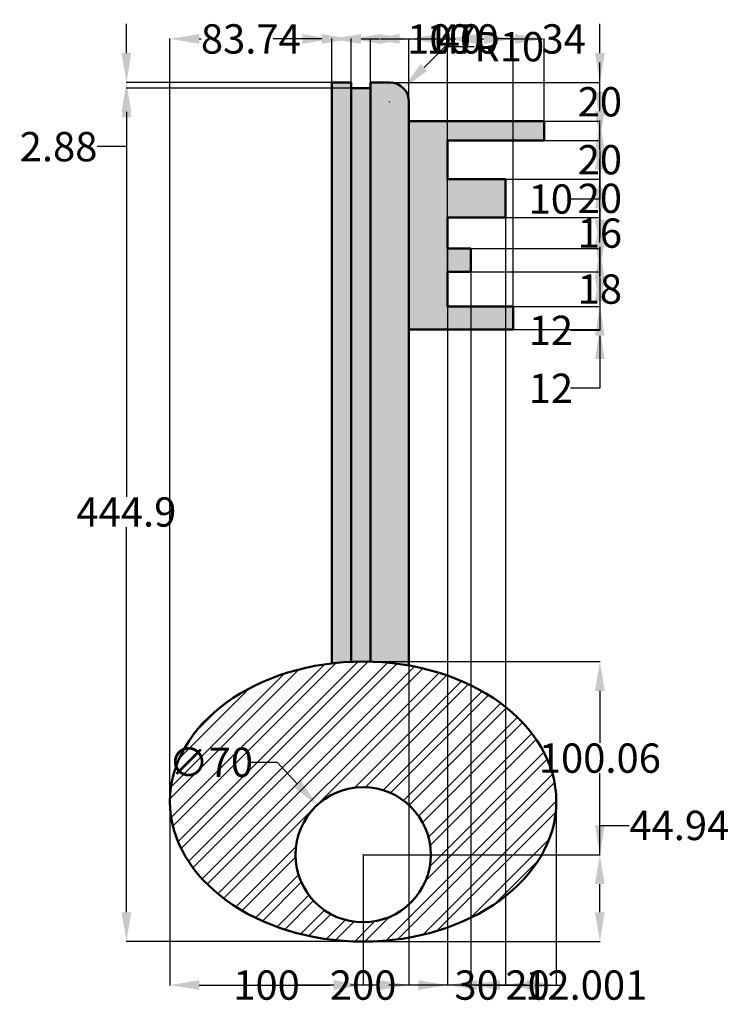
# Model space of a CAD drawing. Units: millimetres. Extents: x 264 to 631, y -41 to 469.
import ezdxf

# ---------------------------------------------------------------- set-up
doc = ezdxf.new("R2010")
doc.units = ezdxf.units.MM
doc.header["$MEASUREMENT"] = 0
for name, color, linetype, lineweight in [('M-DIMS', 2, 'Continuous', 18), ('M-HATC', 252, 'Continuous', 18), ('M-OUTL', 7, 'Continuous', 50)]:
    doc.layers.add(name, color=color, linetype=linetype, lineweight=lineweight)
doc.styles.get("Standard").update_dxf_attribs({"font": 'arial.ttf'})
doc.dimstyles.get("Standard").update_dxf_attribs({"dimtxt": 15.18, "dimasz": 15.18, "dimexe": 0.18, "dimexo": 0.0625, "dimgap": 0.09, "dimtad": 0, "dimtih": 1, "dimtoh": 1, "dimdec": 0, "dimzin": 0, "dimdsep": 46, "dimtxsty": 'Standard', "dimcen": 0.09, "dimadec": 0, "dimazin": 0, "dimtfac": 1, "dimtdec": 0, "dimtofl": 0, "dimtmove": 0, "dimatfit": 3, "dimfxl": 1, "dimtolj": 1, "dimtzin": 0, "dimarcsym": 0})

# ---------------------------------------------------------------- blocks, each defined once
blk = doc.blocks.new('*D1')
at = {"layer": 'Defpoints', "color": 0, "transparency": 16777216}
for p in [(341.801218, 64.408908), (441.8012179999999, 36.853268), (441.8012179999999, -30.641092)]:
    blk.add_point(p, dxfattribs=at)
at = {"layer": 'M-DIMS', "color": 0, "lineweight": -2, "transparency": 16777216}
for p, q in [((341.801218, 64.346408), (341.801218, -30.82109200000001)), ((441.8012179999999, 36.790768), (441.8012179999999, -30.82109200000001)), ((356.981218, -30.641092), (375.6821320518417, -30.641092)), ((426.621218, -30.641092), (407.9203039481583, -30.641092))]:
    blk.add_line(p, q, dxfattribs=at)
at = {"layer": 'M-DIMS', "color": 0, "transparency": 16777216}
for points in [[(356.981218, -28.111092), (356.981218, -33.171092), (341.801218, -30.641092)], [(426.621218, -28.111092), (426.621218, -33.171092), (441.8012179999999, -30.641092)]]:
    blk.add_solid(points, dxfattribs=at)
at = {"layer": 'M-DIMS', "color": 0, "transparency": 16777216, "insert": (391.801218, -30.641092), "char_height": 15.18, "attachment_point": 5}
blk.add_mtext('\\A1;100', dxfattribs=at)
blk = doc.blocks.new('*D2')
at = {"layer": 'Defpoints', "color": 0, "transparency": 16777216}
for p in [(341.801218, 64.408908), (541.801218, 64.408908), (541.801218, -30.641092)]:
    blk.add_point(p, dxfattribs=at)
at = {"layer": 'M-DIMS', "color": 0, "lineweight": -2, "transparency": 16777216}
for p, q in [((341.801218, 64.346408), (341.801218, -30.82109200000001)), ((541.801218, 64.346408), (541.801218, -30.82109200000001)), ((356.981218, -30.641092), (424.8382234570259, -30.641092)), ((526.621218, -30.641092), (458.7642125429741, -30.641092))]:
    blk.add_line(p, q, dxfattribs=at)
at = {"layer": 'M-DIMS', "color": 0, "transparency": 16777216}
for points in [[(356.981218, -28.111092), (356.981218, -33.171092), (341.801218, -30.641092)], [(526.621218, -28.111092), (526.621218, -33.171092), (541.801218, -30.641092)]]:
    blk.add_solid(points, dxfattribs=at)
at = {"layer": 'M-DIMS', "color": 0, "transparency": 16777216, "insert": (441.8012179999999, -30.641092), "char_height": 15.18, "attachment_point": 5}
blk.add_mtext('\\A1;200', dxfattribs=at)
blk = doc.blocks.new('*D3')
at = {"layer": 'Defpoints', "color": 0, "transparency": 16777216}
for p in [(441.8012180000002, 36.85326800000002), (564.3512180000004, 36.85326800000004), (441.8012180000002, -8.091092000000003)]:
    blk.add_point(p, dxfattribs=at)
at = {"layer": 'M-DIMS', "color": 0, "lineweight": -2, "transparency": 16777216}
for p, q in [((564.3512180000004, 36.85326800000004), (564.3512180000004, 52.03326800000004)), ((564.3512180000004, 52.03326800000004), (579.5312180000004, 52.03326800000004)), ((441.8637180000002, 36.85326800000002), (564.5312180000003, 36.85326800000004)), ((564.3512180000004, 7.08890800000002), (564.3512180000004, 21.67326800000003)), ((441.8637180000002, -8.091092000000003), (564.5312180000003, -8.09109199999998))]:
    blk.add_line(p, q, dxfattribs=at)
at = {"layer": 'M-DIMS', "color": 0, "transparency": 16777216}
for points in [[(561.8212180000004, 21.67326800000003), (566.8812180000004, 21.67326800000003), (564.3512180000004, 36.85326800000004)], [(561.8212180000004, 7.088908000000019), (566.8812180000004, 7.088908000000021), (564.3512180000004, -8.09109199999998)]]:
    blk.add_solid(points, dxfattribs=at)
at = {"layer": 'M-DIMS', "color": 0, "transparency": 16777216, "insert": (605.5079847121422, 52.03326799999986), "char_height": 15.18, "attachment_point": 5}
blk.add_mtext('\\A1;44.94', dxfattribs=at)
blk = doc.blocks.new('*D4')
at = {"layer": 'Defpoints', "color": 0, "transparency": 16777216}
for p in [(441.8012180000002, 136.908908), (564.3512180000004, 136.9089080000001), (441.8012180000002, 36.85326800000002)]:
    blk.add_point(p, dxfattribs=at)
at = {"layer": 'M-DIMS', "color": 0, "lineweight": -2, "transparency": 16777216}
for p, q in [((441.8637180000002, 136.908908), (564.5312180000003, 136.9089080000001)), ((564.3512180000004, 121.7289080000001), (564.3512180000004, 94.72158595361535)), ((564.3512180000004, 52.03326800000004), (564.3512180000004, 79.04059004638478)), ((441.8637180000002, 36.85326800000002), (564.5312180000003, 36.85326800000004))]:
    blk.add_line(p, q, dxfattribs=at)
at = {"layer": 'M-DIMS', "color": 0, "transparency": 16777216}
for points in [[(561.8212180000004, 121.7289080000001), (566.8812180000004, 121.7289080000001), (564.3512180000004, 136.9089080000001)], [(561.8212180000004, 52.03326800000004), (566.8812180000004, 52.03326800000004), (564.3512180000004, 36.85326800000004)]]:
    blk.add_solid(points, dxfattribs=at)
at = {"layer": 'M-DIMS', "color": 0, "transparency": 16777216, "insert": (564.3512180000002, 86.88108799999989), "char_height": 15.18, "attachment_point": 5}
blk.add_mtext('\\A1;100.06', dxfattribs=at)
blk = doc.blocks.new('*D5')
at = {"layer": 'Defpoints', "color": 0, "transparency": 16777216}
for p in [(319.2512180000002, 436.7666020000001), (425.5387700000002, 436.7666020000002), (441.8012180000002, -8.091092000000003)]:
    blk.add_point(p, dxfattribs=at)
at = {"layer": 'M-DIMS', "color": 0, "lineweight": -2, "transparency": 16777216}
for p, q in [((425.4762700000002, 436.7666020000002), (319.0712180000002, 436.7666020000001)), ((319.2512180000002, 421.5866020000001), (319.2512180000002, 222.1782529536153)), ((319.2512180000003, 7.08890799999998), (319.2512180000002, 206.4972570463848)), ((441.7387180000002, -8.091092000000003), (319.0712180000003, -8.091092000000023))]:
    blk.add_line(p, q, dxfattribs=at)
at = {"layer": 'M-DIMS', "color": 0, "transparency": 16777216}
for points in [[(316.7212180000002, 421.5866020000001), (321.7812180000001, 421.5866020000001), (319.2512180000002, 436.7666020000001)], [(316.7212180000003, 7.088907999999979), (321.7812180000003, 7.08890799999998), (319.2512180000003, -8.091092000000023)]]:
    blk.add_solid(points, dxfattribs=at)
at = {"layer": 'M-DIMS', "color": 0, "transparency": 16777216, "insert": (319.2512180000002, 214.3377549999999), "char_height": 15.18, "attachment_point": 5}
blk.add_mtext('\\A1;444.9', dxfattribs=at)
blk = doc.blocks.new('*D6')
at = {"layer": 'Defpoints', "color": 0, "transparency": 16777216}
for p in [(425.5387699999999, 459.3166019999999), (425.5387699999999, 436.7666019999999), (341.801218, 64.408908)]:
    blk.add_point(p, dxfattribs=at)
at = {"layer": 'M-DIMS', "color": 0, "lineweight": -2, "transparency": 16777216}
for p, q in [((341.801218, 64.471408), (341.801218, 459.496602)), ((356.981218, 459.3166019999999), (357.9883364283765, 459.3166019999999)), ((410.35877, 459.3166019999999), (409.3516515716234, 459.3166019999999)), ((425.5387699999999, 436.829102), (425.5387699999999, 459.496602))]:
    blk.add_line(p, q, dxfattribs=at)
at = {"layer": 'M-DIMS', "color": 0, "transparency": 16777216}
for points in [[(356.981218, 461.8466019999999), (356.981218, 456.786602), (341.801218, 459.3166019999999)], [(410.35877, 461.8466019999999), (410.35877, 456.786602), (425.5387699999999, 459.3166019999999)]]:
    blk.add_solid(points, dxfattribs=at)
at = {"layer": 'M-DIMS', "color": 0, "transparency": 16777216, "insert": (383.669994, 459.3166019999999), "char_height": 15.18, "attachment_point": 5}
blk.add_mtext('\\A1;83.74', dxfattribs=at)
blk = doc.blocks.new('*D7')
at = {"layer": 'Defpoints', "color": 0, "transparency": 16777216}
for p in [(465.53877, 459.3166019999999), (425.5387699999999, 135.94379), (465.53877, 134.455354)]:
    blk.add_point(p, dxfattribs=at)
at = {"layer": 'M-DIMS', "color": 0, "lineweight": -2, "transparency": 16777216}
for p, q in [((425.5387699999999, 136.00629), (425.5387699999999, 459.4966019999999)), ((440.71877, 459.3166019999999), (450.3587699999999, 459.3166019999999)), ((465.53877, 134.517854), (465.53877, 459.496602)), ((465.53877, 459.3166019999999), (480.71877, 459.3166019999999))]:
    blk.add_line(p, q, dxfattribs=at)
at = {"layer": 'M-DIMS', "color": 0, "transparency": 16777216}
for points in [[(440.71877, 461.8466019999999), (440.71877, 456.786602), (425.5387699999999, 459.3166019999999)], [(450.3587699999999, 461.8466019999999), (450.3587699999999, 456.786602), (465.53877, 459.3166019999999)]]:
    blk.add_solid(points, dxfattribs=at)
at = {"layer": 'M-DIMS', "color": 0, "transparency": 16777216, "insert": (491.9607890995907, 459.3166019999999), "char_height": 15.18, "attachment_point": 5}
blk.add_mtext('\\A1;40', dxfattribs=at)
blk = doc.blocks.new('*D8')
at = {"layer": 'Defpoints', "color": 0, "transparency": 16777216}
for p in [(435.53877, 459.3166019999999), (425.5387699999999, 436.7666019999999), (435.53877, 436.7666019999999)]:
    blk.add_point(p, dxfattribs=at)
at = {"layer": 'M-DIMS', "color": 0, "lineweight": -2, "transparency": 16777216}
for p, q in [((410.35877, 459.3166019999999), (395.17877, 459.3166019999999)), ((425.5387699999999, 436.829102), (425.5387699999999, 459.496602)), ((435.53877, 436.829102), (435.53877, 459.496602)), ((450.71877, 459.3166019999999), (465.8987699999999, 459.3166019999999))]:
    blk.add_line(p, q, dxfattribs=at)
at = {"layer": 'M-DIMS', "color": 0, "transparency": 16777216}
for points in [[(410.35877, 461.8466019999999), (410.35877, 456.786602), (425.5387699999999, 459.3166019999999)], [(450.71877, 461.8466019999999), (450.71877, 456.786602), (435.53877, 459.3166019999999)]]:
    blk.add_solid(points, dxfattribs=at)
at = {"layer": 'M-DIMS', "color": 0, "transparency": 16777216, "insert": (476.1208504911323, 459.3166019999999), "char_height": 15.18, "attachment_point": 5}
blk.add_mtext('\\A1;10', dxfattribs=at)
blk = doc.blocks.new('*D9')
at = {"layer": 'Defpoints', "color": 0, "transparency": 16777216}
for p in [(445.53877, 459.3166019999999), (435.53877, 436.7666019999999), (445.53877, 436.7666019999999)]:
    blk.add_point(p, dxfattribs=at)
at = {"layer": 'M-DIMS', "color": 0, "lineweight": -2, "transparency": 16777216}
for p, q in [((420.3587699999999, 459.3166019999999), (405.17877, 459.3166019999999)), ((435.53877, 436.829102), (435.53877, 459.496602)), ((445.53877, 436.829102), (445.53877, 459.496602)), ((460.7187699999999, 459.3166019999999), (475.89877, 459.3166019999999))]:
    blk.add_line(p, q, dxfattribs=at)
at = {"layer": 'M-DIMS', "color": 0, "transparency": 16777216}
for points in [[(420.3587699999999, 461.8466019999999), (420.3587699999999, 456.786602), (435.53877, 459.3166019999999)], [(460.7187699999999, 461.8466019999999), (460.7187699999999, 456.786602), (445.53877, 459.3166019999999)]]:
    blk.add_solid(points, dxfattribs=at)
at = {"layer": 'M-DIMS', "color": 0, "transparency": 16777216, "insert": (486.1208504911323, 459.3166019999999), "char_height": 15.18, "attachment_point": 5}
blk.add_mtext('\\A1;10', dxfattribs=at)
blk = doc.blocks.new('*D10')
at = {"layer": 'Defpoints', "color": 0, "transparency": 16777216}
for p in [(319.2512180000002, 433.8866020000001), (425.5387700000002, 436.7666020000002), (435.5387700000002, 433.8866020000001)]:
    blk.add_point(p, dxfattribs=at)
at = {"layer": 'M-DIMS', "color": 0, "lineweight": -2, "transparency": 16777216}
for p, q in [((319.2512180000002, 451.9466020000002), (319.2512180000002, 467.1266020000001)), ((425.4762700000002, 436.7666020000002), (319.0712180000002, 436.7666020000001)), ((435.4762700000001, 433.8866020000001), (319.0712180000002, 433.8866020000001)), ((319.2512180000002, 418.7066020000001), (319.2512180000002, 403.5266020000001)), ((319.2512180000002, 403.5266020000001), (304.0712180000002, 403.5266020000001))]:
    blk.add_line(p, q, dxfattribs=at)
at = {"layer": 'M-DIMS', "color": 0, "transparency": 16777216}
for points in [[(316.7212180000003, 451.9466020000002), (321.7812180000002, 451.9466020000002), (319.2512180000002, 436.7666020000001)], [(316.7212180000003, 418.7066020000001), (321.7812180000002, 418.7066020000001), (319.2512180000002, 433.8866020000001)]]:
    blk.add_solid(points, dxfattribs=at)
at = {"layer": 'M-DIMS', "color": 0, "transparency": 16777216, "insert": (284.120890578445, 403.5266019999999), "char_height": 15.18, "attachment_point": 5}
blk.add_mtext('\\A1;2.88', dxfattribs=at)
blk = doc.blocks.new('*D11')
at = {"layer": 'Defpoints', "color": 0, "transparency": 16777216}
for p in [(455.5387700000002, 436.7666020000002), (535.5387700000002, 416.7666020000002), (564.3512180000004, 416.7666020000002)]:
    blk.add_point(p, dxfattribs=at)
at = {"layer": 'M-DIMS', "color": 0, "lineweight": -2, "transparency": 16777216}
for p, q in [((564.3512180000004, 451.9466020000002), (564.3512180000004, 467.1266020000002)), ((455.6012700000002, 436.7666020000002), (564.5312180000005, 436.7666020000002)), ((535.6012700000002, 416.7666020000002), (564.5312180000003, 416.7666020000002)), ((564.3512180000004, 401.5866020000002), (564.3512180000004, 386.4066020000002))]:
    blk.add_line(p, q, dxfattribs=at)
at = {"layer": 'M-DIMS', "color": 0, "transparency": 16777216}
for points in [[(561.8212180000004, 451.9466020000002), (566.8812180000004, 451.9466020000002), (564.3512180000004, 436.7666020000002)], [(561.8212180000004, 401.5866020000002), (566.8812180000004, 401.5866020000002), (564.3512180000004, 416.7666020000002)]]:
    blk.add_solid(points, dxfattribs=at)
at = {"layer": 'M-DIMS', "color": 0, "transparency": 16777216, "insert": (564.3512180000004, 426.7666019999999), "char_height": 15.18, "attachment_point": 5}
blk.add_mtext('\\A1;20', dxfattribs=at)
blk = doc.blocks.new('*D12')
at = {"layer": 'Defpoints', "color": 0, "transparency": 16777216}
for p in [(535.53877, 459.3166019999999), (465.53877, 416.7666019999999), (535.53877, 416.7666019999999)]:
    blk.add_point(p, dxfattribs=at)
at = {"layer": 'M-DIMS', "color": 0, "lineweight": -2, "transparency": 16777216}
for p, q in [((465.53877, 416.8291019999999), (465.53877, 459.496602)), ((480.71877, 459.3166019999999), (489.6643429877216, 459.3166019999999)), ((520.35877, 459.3166019999999), (511.4131970122783, 459.3166019999999)), ((535.53877, 416.8291019999999), (535.53877, 459.496602))]:
    blk.add_line(p, q, dxfattribs=at)
at = {"layer": 'M-DIMS', "color": 0, "transparency": 16777216}
for points in [[(480.71877, 461.8466019999999), (480.71877, 456.786602), (465.53877, 459.3166019999999)], [(520.35877, 461.8466019999999), (520.35877, 456.786602), (535.53877, 459.3166019999999)]]:
    blk.add_solid(points, dxfattribs=at)
at = {"layer": 'M-DIMS', "color": 0, "transparency": 16777216, "insert": (500.5387699999999, 459.3166019999999), "char_height": 15.18, "attachment_point": 5}
blk.add_mtext('\\A1;70', dxfattribs=at)
blk = doc.blocks.new('*D13')
at = {"layer": 'Defpoints', "color": 0, "transparency": 16777216}
for p in [(535.5387700000002, 416.7666020000002), (535.5387700000002, 406.7666020000002), (564.3512180000004, 406.7666020000002)]:
    blk.add_point(p, dxfattribs=at)
at = {"layer": 'M-DIMS', "color": 0, "lineweight": -2, "transparency": 16777216}
for p, q in [((564.3512180000004, 431.9466020000001), (564.3512180000004, 447.1266020000002)), ((535.6012700000002, 416.7666020000002), (564.5312180000003, 416.7666020000002)), ((535.6012700000002, 406.7666020000002), (564.5312180000003, 406.7666020000002)), ((564.3512180000004, 391.5866020000002), (564.3512180000004, 376.4066020000001)), ((564.3512180000004, 376.4066020000001), (549.1712180000005, 376.4066020000001))]:
    blk.add_line(p, q, dxfattribs=at)
at = {"layer": 'M-DIMS', "color": 0, "transparency": 16777216}
for points in [[(561.8212180000004, 431.9466020000001), (566.8812180000004, 431.9466020000001), (564.3512180000004, 416.7666020000002)], [(561.8212180000004, 391.5866020000002), (566.8812180000004, 391.5866020000002), (564.3512180000004, 406.7666020000002)]]:
    blk.add_solid(points, dxfattribs=at)
at = {"layer": 'M-DIMS', "color": 0, "transparency": 16777216, "insert": (538.9491375088681, 376.4066019999999), "char_height": 15.18, "attachment_point": 5}
blk.add_mtext('\\A1;10', dxfattribs=at)
blk = doc.blocks.new('*D14')
at = {"layer": 'Defpoints', "color": 0, "transparency": 16777216}
for p in [(535.5387700000002, 406.7666020000002), (515.5387700000002, 386.7666020000002), (564.3512180000004, 386.7666020000002)]:
    blk.add_point(p, dxfattribs=at)
at = {"layer": 'M-DIMS', "color": 0, "lineweight": -2, "transparency": 16777216}
for p, q in [((564.3512180000004, 421.9466020000002), (564.3512180000004, 437.1266020000001)), ((535.6012700000002, 406.7666020000002), (564.5312180000003, 406.7666020000002)), ((515.6012700000002, 386.7666020000002), (564.5312180000003, 386.7666020000002)), ((564.3512180000004, 371.5866020000001), (564.3512180000004, 356.4066020000002))]:
    blk.add_line(p, q, dxfattribs=at)
at = {"layer": 'M-DIMS', "color": 0, "transparency": 16777216}
for points in [[(561.8212180000004, 421.9466020000002), (566.8812180000004, 421.9466020000002), (564.3512180000004, 406.7666020000002)], [(561.8212180000004, 371.5866020000001), (566.8812180000004, 371.5866020000001), (564.3512180000004, 386.7666020000002)]]:
    blk.add_solid(points, dxfattribs=at)
at = {"layer": 'M-DIMS', "color": 0, "transparency": 16777216, "insert": (564.3512180000004, 396.7666019999999), "char_height": 15.18, "attachment_point": 5}
blk.add_mtext('\\A1;20', dxfattribs=at)
blk = doc.blocks.new('*D15')
at = {"layer": 'Defpoints', "color": 0, "transparency": 16777216}
for p in [(515.5387700000002, 386.7666020000002), (515.5387700000002, 366.7666020000001), (564.3512180000004, 366.7666020000001)]:
    blk.add_point(p, dxfattribs=at)
at = {"layer": 'M-DIMS', "color": 0, "lineweight": -2, "transparency": 16777216}
for p, q in [((564.3512180000004, 401.9466020000002), (564.3512180000004, 417.1266020000002)), ((515.6012700000002, 386.7666020000002), (564.5312180000003, 386.7666020000002)), ((515.6012700000002, 366.7666020000001), (564.5312180000003, 366.7666020000001)), ((564.3512180000004, 351.5866020000001), (564.3512180000004, 336.4066020000001))]:
    blk.add_line(p, q, dxfattribs=at)
at = {"layer": 'M-DIMS', "color": 0, "transparency": 16777216}
for points in [[(561.8212180000004, 401.9466020000002), (566.8812180000004, 401.9466020000002), (564.3512180000004, 386.7666020000002)], [(561.8212180000004, 351.5866020000001), (566.8812180000004, 351.5866020000001), (564.3512180000004, 366.7666020000001)]]:
    blk.add_solid(points, dxfattribs=at)
at = {"layer": 'M-DIMS', "color": 0, "transparency": 16777216, "insert": (564.3512180000004, 376.7666019999999), "char_height": 15.18, "attachment_point": 5}
blk.add_mtext('\\A1;20', dxfattribs=at)
blk = doc.blocks.new('*D16')
at = {"layer": 'Defpoints', "color": 0, "transparency": 16777216}
for p in [(515.5387700000002, 366.7666020000001), (497.5387700000002, 350.7666020000001), (564.3512180000004, 350.7666020000001)]:
    blk.add_point(p, dxfattribs=at)
at = {"layer": 'M-DIMS', "color": 0, "lineweight": -2, "transparency": 16777216}
for p, q in [((564.3512180000004, 381.9466020000001), (564.3512180000004, 397.1266020000001)), ((515.6012700000002, 366.7666020000001), (564.5312180000003, 366.7666020000001)), ((497.6012700000002, 350.7666020000001), (564.5312180000005, 350.7666020000001)), ((564.3512180000004, 335.5866020000001), (564.3512180000004, 320.4066020000001))]:
    blk.add_line(p, q, dxfattribs=at)
at = {"layer": 'M-DIMS', "color": 0, "transparency": 16777216}
for points in [[(561.8212180000004, 381.9466020000001), (566.8812180000004, 381.9466020000001), (564.3512180000004, 366.7666020000001)], [(561.8212180000004, 335.5866020000001), (566.8812180000004, 335.5866020000001), (564.3512180000004, 350.7666020000001)]]:
    blk.add_solid(points, dxfattribs=at)
at = {"layer": 'M-DIMS', "color": 0, "transparency": 16777216, "insert": (564.3512180000004, 358.7666019999999), "char_height": 15.18, "attachment_point": 5}
blk.add_mtext('\\A1;16', dxfattribs=at)
blk = doc.blocks.new('*D17')
at = {"layer": 'Defpoints', "color": 0, "transparency": 16777216}
for p in [(497.5387700000002, 350.7666020000001), (497.5387700000002, 338.7666020000001), (564.3512180000004, 338.7666020000001)]:
    blk.add_point(p, dxfattribs=at)
at = {"layer": 'M-DIMS', "color": 0, "lineweight": -2, "transparency": 16777216}
for p, q in [((564.3512180000004, 365.9466020000001), (564.3512180000004, 381.1266020000001)), ((497.6012700000002, 350.7666020000001), (564.5312180000005, 350.7666020000001)), ((497.6012700000002, 338.7666020000001), (564.5312180000005, 338.7666020000001)), ((564.3512180000004, 323.5866020000001), (564.3512180000004, 308.4066020000001)), ((564.3512180000004, 308.4066020000001), (549.1712180000005, 308.4066020000001))]:
    blk.add_line(p, q, dxfattribs=at)
at = {"layer": 'M-DIMS', "color": 0, "transparency": 16777216}
for points in [[(561.8212180000004, 365.9466020000001), (566.8812180000004, 365.9466020000001), (564.3512180000004, 350.7666020000001)], [(561.8212180000004, 323.5866020000001), (566.8812180000004, 323.5866020000001), (564.3512180000004, 338.7666020000001)]]:
    blk.add_solid(points, dxfattribs=at)
at = {"layer": 'M-DIMS', "color": 0, "transparency": 16777216, "insert": (539.0009110422924, 308.4066019999998), "char_height": 15.18, "attachment_point": 5}
blk.add_mtext('\\A1;12', dxfattribs=at)
blk = doc.blocks.new('*D18')
at = {"layer": 'Defpoints', "color": 0, "transparency": 16777216}
for p in [(497.5387700000002, 338.7666020000001), (519.5387700000002, 320.7666020000001), (564.3512180000004, 320.7666020000001)]:
    blk.add_point(p, dxfattribs=at)
at = {"layer": 'M-DIMS', "color": 0, "lineweight": -2, "transparency": 16777216}
for p, q in [((564.3512180000004, 353.9466020000001), (564.3512180000004, 369.1266020000001)), ((497.6012700000002, 338.7666020000001), (564.5312180000005, 338.7666020000001)), ((519.6012700000002, 320.7666020000001), (564.5312180000003, 320.7666020000001)), ((564.3512180000004, 305.5866020000001), (564.3512180000004, 290.4066020000001))]:
    blk.add_line(p, q, dxfattribs=at)
at = {"layer": 'M-DIMS', "color": 0, "transparency": 16777216}
for points in [[(561.8212180000004, 353.9466020000001), (566.8812180000004, 353.9466020000001), (564.3512180000004, 338.7666020000001)], [(561.8212180000004, 305.5866020000001), (566.8812180000004, 305.5866020000001), (564.3512180000004, 320.7666020000001)]]:
    blk.add_solid(points, dxfattribs=at)
at = {"layer": 'M-DIMS', "color": 0, "transparency": 16777216, "insert": (564.3512180000004, 329.7666019999998), "char_height": 15.18, "attachment_point": 5}
blk.add_mtext('\\A1;18', dxfattribs=at)
blk = doc.blocks.new('*D19')
at = {"layer": 'Defpoints', "color": 0, "transparency": 16777216}
for p in [(519.5387700000002, 320.7666020000001), (519.5387700000002, 308.7666020000001), (564.3512180000004, 308.7666020000001)]:
    blk.add_point(p, dxfattribs=at)
at = {"layer": 'M-DIMS', "color": 0, "lineweight": -2, "transparency": 16777216}
for p, q in [((564.3512180000004, 335.9466020000001), (564.3512180000004, 351.1266020000001)), ((519.6012700000002, 320.7666020000001), (564.5312180000003, 320.7666020000001)), ((519.6012700000002, 308.7666020000001), (564.5312180000003, 308.7666020000001)), ((564.3512180000004, 293.5866020000001), (564.3512180000004, 278.4066020000001)), ((564.3512180000004, 278.4066020000001), (549.1712180000005, 278.4066020000001))]:
    blk.add_line(p, q, dxfattribs=at)
at = {"layer": 'M-DIMS', "color": 0, "transparency": 16777216}
for points in [[(561.8212180000004, 335.9466020000001), (566.8812180000004, 335.9466020000001), (564.3512180000004, 320.7666020000001)], [(561.8212180000004, 293.5866020000001), (566.8812180000004, 293.5866020000001), (564.3512180000004, 308.7666020000001)]]:
    blk.add_solid(points, dxfattribs=at)
at = {"layer": 'M-DIMS', "color": 0, "transparency": 16777216, "insert": (539.0009110422924, 278.4066019999999), "char_height": 15.18, "attachment_point": 5}
blk.add_mtext('\\A1;12', dxfattribs=at)
blk = doc.blocks.new('*D20')
at = {"layer": 'Defpoints', "color": 0, "transparency": 16777216}
for p in [(485.5373089999999, 320.766602), (465.53877, 308.766602), (485.5373089999999, -30.641092)]:
    blk.add_point(p, dxfattribs=at)
at = {"layer": 'M-DIMS', "color": 0, "lineweight": -2, "transparency": 16777216}
for p, q in [((485.5373089999999, 320.704102), (485.5373089999999, -30.82109200000002)), ((465.53877, 308.704102), (465.53877, -30.82109200000002)), ((450.3587699999999, -30.641092), (435.17877, -30.641092)), ((500.717309, -30.641092), (515.897309, -30.641092))]:
    blk.add_line(p, q, dxfattribs=at)
at = {"layer": 'M-DIMS', "color": 0, "transparency": 16777216}
for points in [[(450.3587699999999, -28.111092), (450.3587699999999, -33.171092), (465.53877, -30.641092)], [(500.717309, -28.111092), (500.717309, -33.171092), (485.5373089999999, -30.641092)]]:
    blk.add_solid(points, dxfattribs=at)
at = {"layer": 'M-DIMS', "color": 0, "transparency": 16777216, "insert": (526.9632980859482, -30.641092), "char_height": 15.18, "attachment_point": 5}
blk.add_mtext('\\A1;20', dxfattribs=at)
blk = doc.blocks.new('*D21')
at = {"layer": 'Defpoints', "color": 0, "transparency": 16777216}
for p in [(485.53877, 366.766602), (515.53877, 366.766602), (515.53877, -30.641092)]:
    blk.add_point(p, dxfattribs=at)
at = {"layer": 'M-DIMS', "color": 0, "lineweight": -2, "transparency": 16777216}
for p, q in [((485.53877, 366.704102), (485.53877, -30.82109200000002)), ((515.53877, 366.704102), (515.53877, -30.82109200000002)), ((470.3587699999999, -30.641092), (455.17877, -30.641092)), ((530.71877, -30.641092), (545.89877, -30.641092))]:
    blk.add_line(p, q, dxfattribs=at)
at = {"layer": 'M-DIMS', "color": 0, "transparency": 16777216}
for points in [[(470.3587699999999, -28.111092), (470.3587699999999, -33.171092), (485.53877, -30.641092)], [(530.71877, -28.111092), (530.71877, -33.171092), (515.53877, -30.641092)]]:
    blk.add_solid(points, dxfattribs=at)
at = {"layer": 'M-DIMS', "color": 0, "transparency": 16777216, "insert": (500.5387699999999, -30.641092), "char_height": 15.18, "attachment_point": 5}
blk.add_mtext('\\A1;30', dxfattribs=at)
blk = doc.blocks.new('*D22')
at = {"layer": 'Defpoints', "color": 0, "transparency": 16777216}
for p in [(485.5373089999999, 338.766602), (497.5387699999999, 338.766602), (497.5387699999999, -30.641092)]:
    blk.add_point(p, dxfattribs=at)
at = {"layer": 'M-DIMS', "color": 0, "lineweight": -2, "transparency": 16777216}
for p, q in [((485.5373089999999, 338.704102), (485.5373089999999, -30.82109200000002)), ((497.5387699999999, 338.704102), (497.5387699999999, -30.82109200000002)), ((470.3573089999999, -30.641092), (455.177309, -30.641092)), ((512.71877, -30.641092), (527.8987699999999, -30.641092))]:
    blk.add_line(p, q, dxfattribs=at)
at = {"layer": 'M-DIMS', "color": 0, "transparency": 16777216}
for points in [[(470.3573089999999, -28.111092), (470.3573089999999, -33.171092), (485.5373089999999, -30.641092)], [(512.71877, -28.111092), (512.71877, -33.171092), (497.5387699999999, -30.641092)]]:
    blk.add_solid(points, dxfattribs=at)
at = {"layer": 'M-DIMS', "color": 0, "transparency": 16777216, "insert": (557.3184766848567, -30.641092), "char_height": 15.18, "attachment_point": 5}
blk.add_mtext('\\A1;12.001', dxfattribs=at)
blk = doc.blocks.new('*D23')
at = {"layer": 'Defpoints', "color": 0, "transparency": 16777216}
for p in [(519.53877, 459.3166019999999), (485.5373089999999, 320.766602), (519.53877, 320.766602)]:
    blk.add_point(p, dxfattribs=at)
at = {"layer": 'M-DIMS', "color": 0, "lineweight": -2, "transparency": 16777216}
for p, q in [((485.5373089999999, 320.829102), (485.5373089999999, 459.496602)), ((500.717309, 459.3166019999999), (504.3587699999999, 459.3166019999999)), ((519.53877, 320.829102), (519.53877, 459.496602)), ((519.53877, 459.3166019999999), (534.71877, 459.3166019999999))]:
    blk.add_line(p, q, dxfattribs=at)
at = {"layer": 'M-DIMS', "color": 0, "transparency": 16777216}
for points in [[(500.717309, 461.8466019999999), (500.717309, 456.786602), (485.5373089999999, 459.3166019999999)], [(504.3587699999999, 461.8466019999999), (504.3587699999999, 456.786602), (519.53877, 459.3166019999999)]]:
    blk.add_solid(points, dxfattribs=at)
at = {"layer": 'M-DIMS', "color": 0, "transparency": 16777216, "insert": (545.6449705457024, 459.3166019999999), "char_height": 15.18, "attachment_point": 5}
blk.add_mtext('\\A1;34', dxfattribs=at)
blk = doc.blocks.new('*D24')
at = {"layer": 'Defpoints', "color": 0, "transparency": 16777216}
for p in [(417.992738, 62.50782499999994), (465.609698, 11.198711)]:
    blk.add_point(p, dxfattribs=at)
at = {"layer": 'M-DIMS', "color": 0, "lineweight": -2, "transparency": 16777216}
for p, q in [((382.1605823302733, 84.76132059492565), (397.3405823302733, 84.7613205949256)), ((397.3405823302733, 84.7613205949256), (407.6666601651367, 73.6345727974628)), ((441.7112180000001, 36.85326800000002), (441.8912180000001, 36.85326799999999)), ((441.801218, 36.76326800000007), (441.801218, 36.94326800000002))]:
    blk.add_line(p, q, dxfattribs=at)
at = {"layer": 'M-DIMS', "color": 0, "transparency": 16777216}
blk.add_solid([(409.5211181313804, 75.35558576994), (405.8122021988928, 71.91355982498558), (417.992738, 62.50782499999994)], dxfattribs=at)
at = {"layer": 'M-DIMS', "color": 0, "transparency": 16777216, "insert": (362.9661484967126, 84.7613205949256), "char_height": 15.18, "attachment_point": 5}
blk.add_mtext('\\A1;∅70', dxfattribs=at)
blk = doc.blocks.new('*D25')
at = {"layer": 'Defpoints', "color": 0, "transparency": 16777216}
for p in [(462.6097539999999, 433.8377539999998), (455.5387699999998, 426.7666019999998)]:
    blk.add_point(p, dxfattribs=at)
at = {"layer": 'M-DIMS', "color": 0, "lineweight": -2, "transparency": 16777216}
for p, q in [((484.0772608513154, 455.3057708993019), (473.3435074256576, 444.5717624496508)), ((499.2572608513153, 455.3057708993019), (484.0772608513154, 455.3057708993019)), ((455.4487699999999, 426.7666019999999), (455.6287699999997, 426.7666019999999)), ((455.5387699999998, 426.6766019999999), (455.5387699999998, 426.8566019999998))]:
    blk.add_line(p, q, dxfattribs=at)
at = {"layer": 'M-DIMS', "color": 0, "transparency": 16777216}
blk.add_solid([(471.5545060173824, 446.3607213539272), (475.1325088339327, 442.7828035453745), (462.6097539999999, 433.8377539999998)], dxfattribs=at)
at = {"layer": 'M-DIMS', "color": 0, "transparency": 16777216, "insert": (517.45764284313, 455.3057708993019), "char_height": 15.18, "attachment_point": 5}
blk.add_mtext('\\A1;R10', dxfattribs=at)

msp = doc.modelspace()

# ---------------------------------------------------------------- hatches: boundary and pattern name
at = {"layer": 'M-HATC'}
h = msp.add_hatch(color=256, dxfattribs=at)
h.dxf.hatch_style = 1
edge = h.paths.add_edge_path()
edge.add_line((435.5387696480566, 436.7666020425589), (425.5387696480566, 436.7666020425589))
edge.add_line((425.5387696480566, 436.7666020425589), (425.5387696480566, 416.7666020425589))
edge.add_line((425.5387696480566, 416.7666020425589), (425.5387696480566, 135.9437904173123))
edge.add_ellipse((441.8012176761867, 64.40890787977284), major_axis=(100, 0), ratio=0.725, start_angle=94.94653596688238, end_angle=102.80770862923009, ccw=False)
edge.add_line((435.5387696480566, 136.766602042559), (435.5387696480566, 436.7666020425589))
edge = h.paths.add_edge_path()
edge.add_arc((455.5387696480566, 426.7666020425589), 9.999999999999998, 0, 90)
edge.add_line((455.5387696480566, 436.7666020425589), (445.5387696480566, 436.7666020425589))
edge.add_line((445.5387696480566, 436.7666020425589), (445.5387696480566, 433.8866020425589))
edge.add_line((445.5387696480566, 433.8866020425589), (445.5387696480566, 136.8582514892977))
edge.add_ellipse((441.8012176761867, 64.40890787977284), major_axis=(100, 0), ratio=0.725, start_angle=71.37371239801098, end_angle=87.04681544636048, ccw=False)
edge.add_line((465.5387696480566, 134.8367103390462), (465.5387696480566, 426.7666020425589))
h.paths.add_polyline_path([(485.5387696480566, 406.7666020425589), (535.5387696480566, 406.7666020425589), (535.5387696480566, 416.7666020425589), (525.5387696480566, 416.7666020425589), (485.5387696480566, 416.7666020425589), (465.5387696480566, 416.7666020425589), (465.5387696480566, 308.7666020425589), (519.5387696480565, 308.7666020425589), (519.5387696480565, 320.7666020425589), (485.5373090045459, 320.7666020425589), (485.5373090045459, 338.7666020425589), (497.5387696480566, 338.7666020425589), (497.5387696480566, 350.7666020425594), (485.5387696480567, 350.7666020425594), (485.5387696480566, 366.7666020425589), (515.5387696480566, 366.7666020425589), (515.5387696480566, 386.7666020425589), (485.5387696480566, 386.7666020425589)])
h = msp.add_hatch(color=256, dxfattribs=at)
h.dxf.hatch_style = 1
edge = h.paths.add_edge_path()
edge.add_line((445.5387696480566, 433.8866020425589), (435.5387696480566, 433.8866020425589))
edge.add_line((435.5387696480566, 433.8866020425589), (435.5387696480566, 136.7666020425589))
edge.add_ellipse((441.8012176761867, 64.40890787977284), major_axis=(100, 0), ratio=0.725, start_angle=87.04681544636048, end_angle=94.94653596688238, ccw=False)
edge.add_line((445.5387696480566, 136.8582514892977), (445.5387696480566, 433.8866020425589))
h = msp.add_hatch(dxfattribs=at)
h.set_pattern_fill('ANSI32', color=256, scale=30)
h.set_pattern_definition([(45, (0, 0), (-7.95495128834866, 7.95495128834866), []), (45, (5.30330085, 0), (-7.95495128834866, 7.95495128834866), [])])
edge = h.paths.add_edge_path()
edge.add_ellipse((441.8012176761867, 64.40890787977284), major_axis=(100, 0), ratio=0.725, start_angle=102.8077086292301, end_angle=431.3737123980109)
edge.add_ellipse((441.8012176761867, 64.40890787977284), major_axis=(100, 0), ratio=0.725, start_angle=71.37371239801092, end_angle=87.04681544636054)
edge.add_ellipse((441.8012176761867, 64.40890787977284), major_axis=(100, 0), ratio=0.725, start_angle=87.04681544636054, end_angle=94.94653596688241)
edge.add_ellipse((441.8012176761867, 64.40890787977284), major_axis=(100, 0), ratio=0.725, start_angle=94.94653596688241, end_angle=102.8077086292301)
h.paths.add_polyline_path([(476.8012176761867, 36.8532675849147, -1), (406.8012176761867, 36.8532675849147, -1)], flags=16)

# ---------------------------------------------------------------- linework, layer by layer
at = {"layer": 'M-OUTL'}
for p, q in [((425.5387696480566, 436.7666020425589), (425.5387696480566, 416.7666020425589)), ((425.5387696480566, 436.7666020425589), (425.5387696480566, 416.7666020425589)), ((465.5387696480566, 416.7666020425589), (485.5387696480566, 416.7666020425589)), ((485.5387696480566, 416.7666020425589), (535.5387696480566, 416.7666020425589)), ((535.5387696480566, 416.7666020425589), (525.5387696480566, 416.7666020425589)), ((535.5387696480566, 416.7666020425589), (535.5387696480566, 406.7666020425589)), ((535.5387696480566, 406.7666020425589), (485.5387696480566, 406.7666020425589)), ((485.5387696480566, 406.7666020425589), (485.5387696480566, 386.7666020425589)), ((485.5387696480566, 386.7666020425589), (515.5387696480566, 386.7666020425589)), ((515.5387696480566, 386.7666020425589), (515.5387696480566, 366.7666020425589)), ((515.5387696480566, 366.7666020425589), (485.5387696480566, 366.7666020425589)), ((485.5387696480566, 366.7666020425589), (485.5387696480567, 350.7666020425594)), ((485.5387696480567, 350.7666020425594), (497.5387696480566, 350.7666020425594)), ((497.5387696480566, 350.7666020425594), (497.5387696480566, 338.7666020425589)), ((497.5387696480566, 338.7666020425589), (485.5373090045459, 338.7666020425589)), ((485.5373090045459, 338.7666020425589), (485.5373090045459, 320.7666020425589)), ((510.5387696480566, 320.7666020425589), (485.5373090045459, 320.7666020425589)), ((485.5373090045459, 320.7666020425589), (519.5387696480565, 320.7666020425589)), ((519.5387696480565, 320.7666020425589), (519.5387696480565, 308.7666020425589)), ((519.5387696480565, 308.7666020425589), (465.5387696480566, 308.7666020425589)), ((517.0680484260165, 308.7666020425589), (517.0680484260165, 308.7666020425589)), ((425.5387696480566, 136.4031912327888), (425.5387696480566, 135.9437904173123))]:
    msp.add_line(p, q, dxfattribs=at)
for points in [[(435.5387696480566, 436.7666020425589), (425.5387696480566, 436.7666020425589), (425.5387696480566, 136.4031912327888)], [(435.5387696480566, 136.7666020425589), (435.5387696480566, 436.7666020425589), (435.5387696480566, 433.8866020425589), (445.5387696480566, 433.8866020425589)]]:
    msp.add_lwpolyline(points, dxfattribs=at)
msp.add_lwpolyline([(445.5387696480566, 136.7342245045231), (445.5387696480566, 433.8866020425589), (445.5387696480566, 436.7666020425589), (455.5387696480566, 436.7666020425589), (455.5387696480566, 436.7666020425589, -0.4142135623730951), (465.5387696480566, 426.7666020425589), (465.5387696480566, 134.45535355176)], format="xyb", dxfattribs=at)
msp.add_circle((441.8012176761867, 36.8532675849147), 35, dxfattribs=at)
msp.add_ellipse((441.8012176761867, 64.40890787977284), major_axis=(100, 0), ratio=0.725, dxfattribs=at)

# ---------------------------------------------------------------- dimensions: what is measured, and where the dimension line sits
at = {"layer": 'M-DIMS'}
for base, p1, p2, override, picture, middle in [((425.5387699999999, 459.3166019999999), (341.801218, 64.408908), (425.5387699999999, 436.7666019999999), {"dimdec": 2, "dimlfac": 1, "dimrnd": 0, "dimzin": 0, "dimdsep": 46, "dimlunit": 2}, '*D6', (383.669994, 459.3166019999999)), ((435.53877, 459.3166019999999), (425.5387699999999, 436.7666019999999), (435.53877, 436.7666019999999), {"dimdec": 0, "dimlfac": 1, "dimrnd": 0, "dimzin": 0, "dimdsep": 46, "dimlunit": 2}, '*D8', (476.1208504911323, 459.3166019999999)), ((445.53877, 459.3166019999999), (435.53877, 436.7666019999999), (445.53877, 436.7666019999999), {"dimdec": 0, "dimlfac": 1, "dimrnd": 0, "dimzin": 0, "dimdsep": 46, "dimlunit": 2}, '*D9', (486.1208504911323, 459.3166019999999)), ((465.53877, 459.3166019999999), (425.5387699999999, 135.94379), (465.53877, 134.455354), {"dimdec": 0, "dimlfac": 1, "dimrnd": 0, "dimzin": 0, "dimdsep": 46, "dimlunit": 2}, '*D7', (491.9607890995907, 459.3166019999999)), ((535.53877, 459.3166019999999), (465.53877, 416.7666019999999), (535.53877, 416.7666019999999), {"dimdec": 0, "dimlfac": 1, "dimrnd": 0, "dimzin": 0, "dimdsep": 46, "dimlunit": 2}, '*D12', (500.5387699999999, 459.3166019999999)), ((519.53877, 459.3166019999999), (485.5373089999999, 320.766602), (519.53877, 320.766602), {"dimdec": 0, "dimlfac": 1, "dimrnd": 0, "dimzin": 0, "dimdsep": 46, "dimlunit": 2}, '*D23', (545.6449705457024, 459.3166019999999)), ((515.53877, -30.641092), (485.53877, 366.766602), (515.53877, 366.766602), {"dimdec": 0, "dimlfac": 1, "dimrnd": 0, "dimzin": 0, "dimdsep": 46, "dimlunit": 2}, '*D21', (500.5387699999999, -30.641092)), ((497.5387699999999, -30.641092), (485.5373089999999, 338.766602), (497.5387699999999, 338.766602), {"dimdec": 3, "dimlfac": 1, "dimrnd": 0, "dimzin": 0, "dimdsep": 46, "dimlunit": 2}, '*D22', (557.3184766848567, -30.641092)), ((485.5373089999999, -30.641092), (465.53877, 308.766602), (485.5373089999999, 320.766602), {"dimdec": 0, "dimlfac": 1, "dimrnd": 0, "dimzin": 0, "dimdsep": 46, "dimlunit": 2}, '*D20', (526.9632980859482, -30.641092)), ((441.8012179999999, -30.641092), (341.801218, 64.408908), (441.8012179999999, 36.853268), {"dimdec": 0, "dimlfac": 1, "dimrnd": 0, "dimzin": 0, "dimdsep": 46, "dimlunit": 2}, '*D1', (391.801218, -30.641092)), ((541.801218, -30.641092), (341.801218, 64.408908), (541.801218, 64.408908), {"dimdec": 0, "dimlfac": 1, "dimrnd": 0, "dimzin": 0, "dimdsep": 46, "dimlunit": 2}, '*D2', (441.8012179999999, -30.641092))]:
    dim = msp.add_linear_dim(base=base, p1=p1, p2=p2, dimstyle='Standard', override=override, dxfattribs=at)
    dim.commit()
    dim.dimension.update_dxf_attribs({"geometry": picture, "text_midpoint": middle})
for base, p1, p2, override, picture, middle in [((319.2512180000002, 433.8866020000001), (425.5387699999999, 436.7666019999999), (435.53877, 433.886602), {"dimdec": 2, "dimlfac": 1, "dimrnd": 0, "dimzin": 0, "dimdsep": 46, "dimlunit": 2}, '*D10', (284.120890578445, 403.5266019999999)), ((564.3512180000004, 416.7666020000002), (455.5387699999999, 436.7666019999999), (535.53877, 416.7666019999999), {"dimdec": 0, "dimlfac": 1, "dimrnd": 0, "dimzin": 0, "dimdsep": 46, "dimlunit": 2}, '*D11', (564.3512180000004, 426.7666019999999)), ((564.3512180000004, 406.7666020000002), (535.53877, 416.7666019999999), (535.53877, 406.7666019999999), {"dimdec": 0, "dimlfac": 1, "dimrnd": 0, "dimzin": 0, "dimdsep": 46, "dimlunit": 2}, '*D13', (538.9491375088681, 376.4066019999999)), ((319.2512180000002, 436.7666020000001), (441.8012179999999, -8.091092), (425.5387699999999, 436.7666019999999), {"dimdec": 1, "dimlfac": 1, "dimrnd": 0, "dimzin": 0, "dimdsep": 46, "dimlunit": 2}, '*D5', (319.2512180000002, 214.3377549999999)), ((564.3512180000004, 386.7666020000002), (535.53877, 406.7666019999999), (515.53877, 386.766602), {"dimdec": 0, "dimlfac": 1, "dimrnd": 0, "dimzin": 0, "dimdsep": 46, "dimlunit": 2}, '*D14', (564.3512180000004, 396.7666019999999)), ((564.3512180000004, 366.7666020000001), (515.53877, 386.766602), (515.53877, 366.766602), {"dimdec": 0, "dimlfac": 1, "dimrnd": 0, "dimzin": 0, "dimdsep": 46, "dimlunit": 2}, '*D15', (564.3512180000004, 376.7666019999999)), ((564.3512180000004, 350.7666020000001), (515.53877, 366.766602), (497.5387699999999, 350.766602), {"dimdec": 0, "dimlfac": 1, "dimrnd": 0, "dimzin": 0, "dimdsep": 46, "dimlunit": 2}, '*D16', (564.3512180000004, 358.7666019999999)), ((564.3512180000004, 338.7666020000001), (497.5387699999999, 350.766602), (497.5387699999999, 338.766602), {"dimdec": 0, "dimlfac": 1, "dimrnd": 0, "dimzin": 0, "dimdsep": 46, "dimlunit": 2}, '*D17', (539.0009110422924, 308.4066019999998)), ((564.3512180000004, 320.7666020000001), (497.5387699999999, 338.766602), (519.53877, 320.766602), {"dimdec": 0, "dimlfac": 1, "dimrnd": 0, "dimzin": 0, "dimdsep": 46, "dimlunit": 2}, '*D18', (564.3512180000004, 329.7666019999998)), ((564.3512180000004, 308.7666020000001), (519.53877, 320.766602), (519.53877, 308.766602), {"dimdec": 0, "dimlfac": 1, "dimrnd": 0, "dimzin": 0, "dimdsep": 46, "dimlunit": 2}, '*D19', (539.0009110422924, 278.4066019999999)), ((564.3512180000004, 136.9089080000001), (441.8012179999999, 36.853268), (441.8012179999999, 136.908908), {"dimdec": 2, "dimlfac": 1, "dimrnd": 0, "dimzin": 0, "dimdsep": 46, "dimlunit": 2}, '*D4', (564.3512180000002, 86.88108799999989)), ((564.3512180000004, 36.85326800000004), (441.8012179999999, -8.091092), (441.8012179999999, 36.853268), {"dimdec": 2, "dimlfac": 1, "dimrnd": 0, "dimzin": 0, "dimdsep": 46, "dimlunit": 2}, '*D3', (605.5079847121422, 52.03326799999986))]:
    dim = msp.add_linear_dim(base=base, p1=p1, p2=p2, angle=90, dimstyle='Standard', override=override, dxfattribs=at)
    dim.commit()
    dim.dimension.update_dxf_attribs({"geometry": picture, "text_midpoint": middle})
dim = msp.add_radius_dim(center=(455.5387699999998, 426.7666019999998), mpoint=(462.6097539999999, 433.8377539999998), dimstyle='Standard', override={"dimdec": 0, "dimlfac": 1, "dimrnd": 0, "dimzin": 0, "dimdsep": 46, "dimlunit": 2}, dxfattribs=at)
dim.commit()
dim.dimension.update_dxf_attribs({"geometry": '*D25', "text_midpoint": (517.45764284313, 455.3057708993019)})
dim = msp.add_diameter_dim_2p(p1=(465.609698, 11.198711), p2=(417.992738, 62.50782499999994), dimstyle='Standard', override={"dimdec": 0, "dimlfac": 1, "dimrnd": 0, "dimzin": 0, "dimdsep": 46, "dimlunit": 2}, dxfattribs=at)
dim.commit()
dim.dimension.update_dxf_attribs({"geometry": '*D24', "text_midpoint": (362.9661484967126, 84.7613205949256), "dimtype": 163})

doc.saveas('drawing.dxf')
